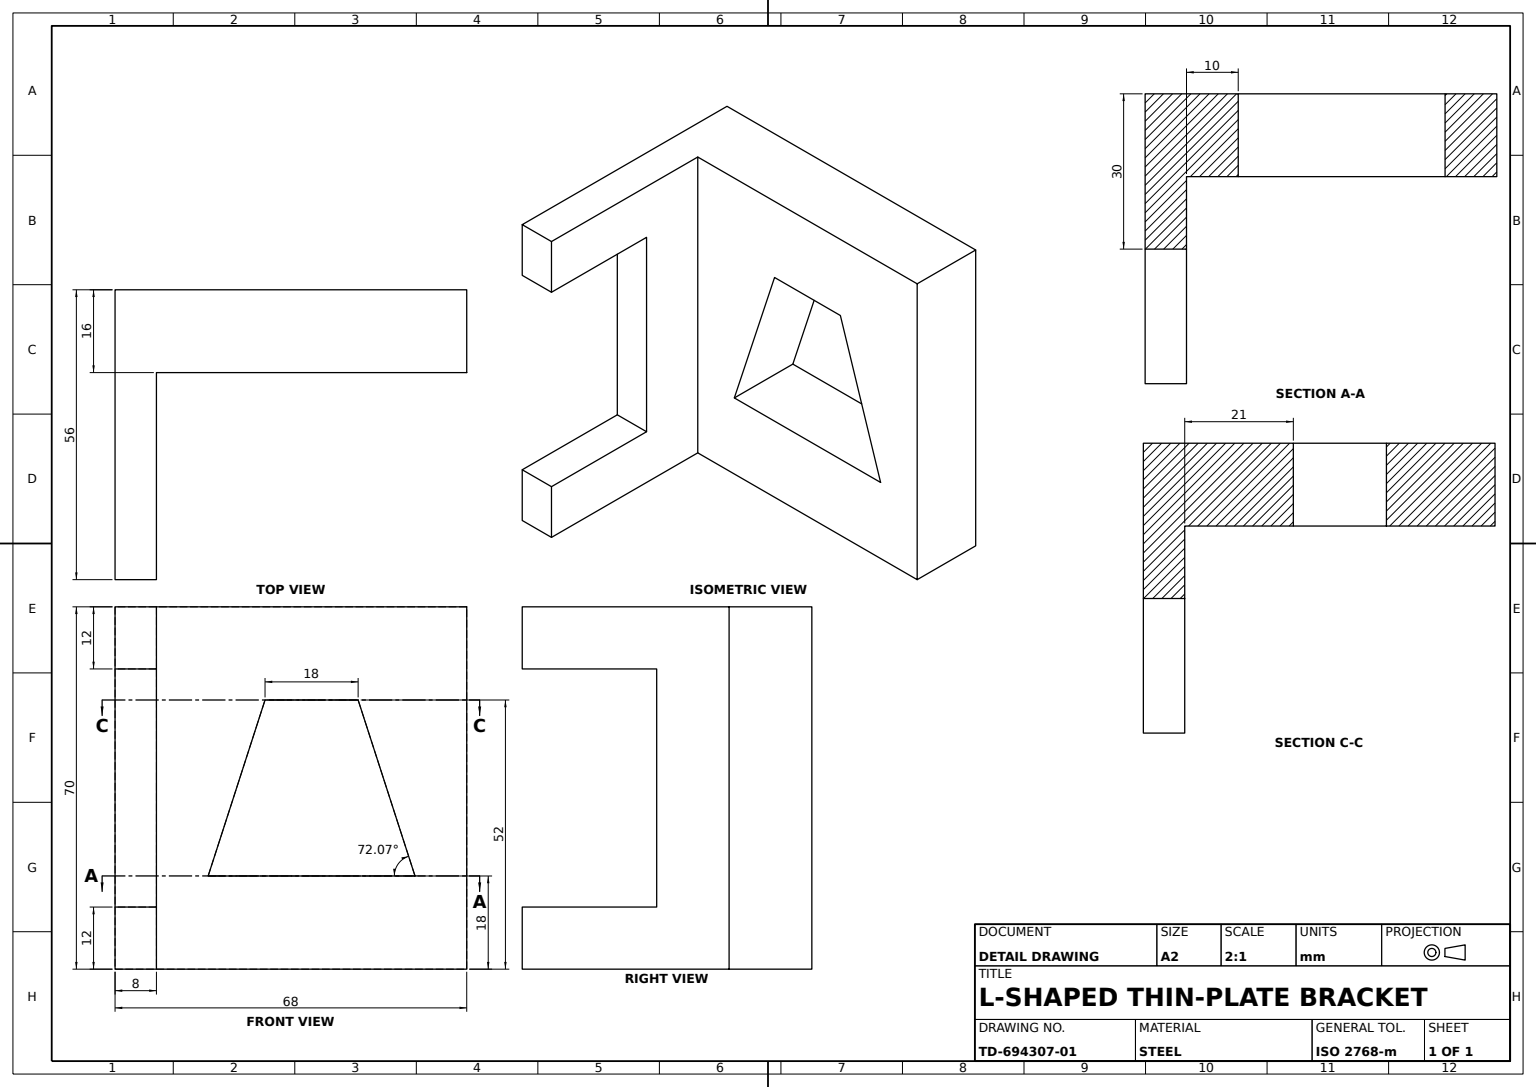
SolidWorks part; units mm, degrees
material "Plain Carbon Steel"
ref_plane "Front Plane" through (0, 0, 0) normal (0, 0, 1) x (1, 0, 0)
ref_plane "Top Plane" through (0, 0, 0) normal (0, 1, 0) x (1, 0, 0)
ref_plane "Right Plane" through (0, 0, 0) normal (1, 0, 0) x (0, 0, -1)
sketch "Base Plate Sketch" plane through (0, 0, 0) normal (0, 0, 1) x (1, 0, 0)
  line L0 (0, 0) -> (68, 0)
  line L1 (68, 0) -> (68, 70)
  line L2 (68, 70) -> (0, 70)
  line L3 (0, 70) -> (0, 0)
  dimension "D1" = 68
  dimension "D2" = 70
extrude "Base Plate 16mm" add sketch "Base Plate Sketch" along normal blind 16
sketch "Side Flange Sketch" plane through (0, 0, 0) normal (-1, 0, 0) x (0, 0, 1)
  line L0 (16, 70) -> (56, 70)
  line L1 (56, 70) -> (56, 58)
  line L2 (56, 58) -> (30, 58)
  line L3 (16, 0) -> (56, 0)
  line L4 (56, 0) -> (56, 12)
  line L5 (56, 12) -> (30, 12)
  line L6 (30, 12) -> (30, 58)
  line L7 (0, 70) -> (0, 0) construction
  line L8 (16, 0) -> (0, 0) construction
  line L11 (0, 70) -> (0, 0)
  line L12 (0, 0) -> (16, 0)
  line L13 (16, 0) -> (16, 70)
  line L14 (16, 70) -> (0, 70)
  line L15 (0, 70) -> (0, 0)
  line L16 (0, 0) -> (16, 0)
  line L18 (16, 70) -> (0, 70)
  dimension "D1" = 0
  dimension "D2" = 30
  dimension "D3" = 56
  dimension "D4" = 12
extrude "C Side Flange 8mm" add sketch "Side Flange Sketch" against normal blind 8
sketch "Window Sketch" plane through (0, 0, 16) normal (0, 0, 1) x (1, 0, 0)
  line L0 (8, 70) -> (8, 0) construction
  line L1 (68, 70) -> (8, 70) construction
  line L3 (58, 18) -> (18, 18)
  line L6 (29, 52) -> (38, 52)
  line L7 (38, 52) -> (47, 52)
  line L8 (47, 52) -> (58, 18)
  line L9 (18, 18) -> (29, 52)
  dimension "D1" = 10
  dimension "D2" = 21
  dimension "D3" = 30
  dimension "D4" = 18
  dimension "D5" = 52
extrude "Window Cut-Out" cut sketch "Window Sketch" against normal blind 18
